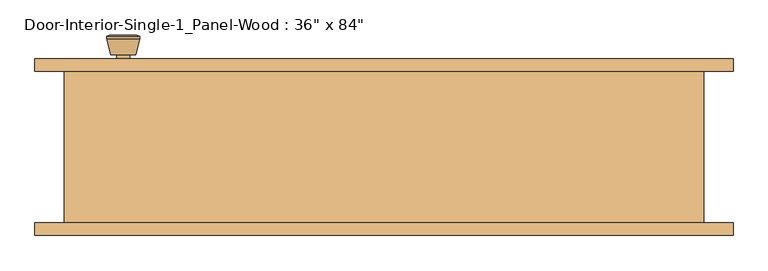
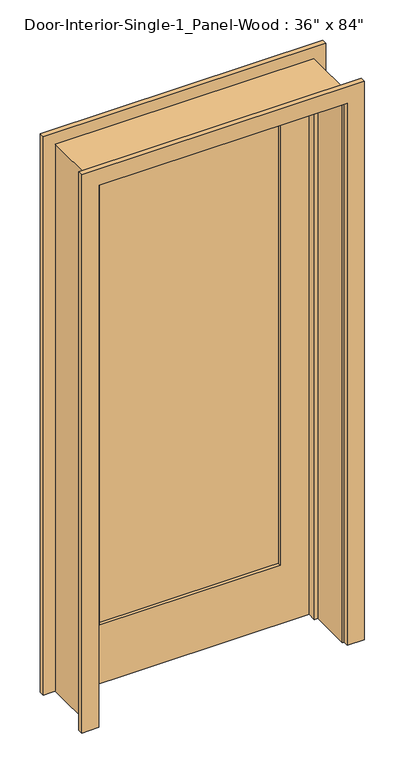
"""IFC4 building model written with IfcOpenShell, lengths in millimetres: door geometry."""

from ifc_helpers import new_model, si_unit, point, frame, frame_2d, origin, place, context, project, spatial, polyline, circle_curve, trimmed, segment, composite_curve, outline, extrude, faceted_brep, source, transform, mapped, element, save
from ifc_brep_helpers import plane_surface, cylinder_surface, revolved_surface, advanced_brep


def door_3b97b8e7(model_context):
    return source(origin(), model_context, "Body", "SolidModel", [
        advanced_brep(
        [(-393.7, 70.2, 914.4), (-383.7, 70.2, 914.4), (-403.7, 70.2, 914.4), (-373.2241324, 21.2, 914.4), (-393.7, 21.2, 914.4), (-414.1758676, 21.2, 914.4), (-368.7, 23.0278681, 914.4), (-418.7, 23.0278681, 914.4), (-368.7, 26.4915463, 914.4), (-418.7, 26.4915463, 914.4), (-375.063764, 51.2, 914.4), (-412.336236, 51.2, 914.4), (-383.7, 51.2, 914.4), (-403.7, 51.2, 914.4)],
        [
            (0, 1),
            (1, 2, circle_curve(frame((-393.7, 70.2, 914.4), z_axis=(0.0, 1.0, 0.0), x_axis=(-1.0, 0.0, 0.0)), 10.0)),
            (2, 0),
            (2, 1, circle_curve(frame((-393.7, 70.2, 914.4), z_axis=(0.0, 1.0, 0.0), x_axis=(-1.0, 0.0, 0.0)), 10.0)),
            (3, 4),
            (4, 5),
            (5, 3, circle_curve(frame((-393.7, 21.2, 914.4), z_axis=(0.0, -1.0, 0.0), x_axis=(-1.0, 0.0, 0.0)), 20.4758676)),
            (3, 5, circle_curve(frame((-393.7, 21.2, 914.4), z_axis=(0.0, -1.0, 0.0), x_axis=(-1.0, 0.0, 0.0)), 20.4758676)),
            (6, 3),
            (5, 7),
            (7, 6, circle_curve(frame((-393.7, 23.0278681, 914.4), z_axis=(0.0, -1.0, 0.0), x_axis=(-1.0, 0.0, 0.0)), 25.0)),
            (6, 7, circle_curve(frame((-393.7, 23.0278681, 914.4), z_axis=(0.0, -1.0, 0.0), x_axis=(-1.0, 0.0, 0.0)), 25.0)),
            (8, 6),
            (7, 9),
            (9, 8, circle_curve(frame((-393.7, 26.4915463, 914.4), z_axis=(0.0, -1.0, 0.0), x_axis=(-1.0, 0.0, 0.0)), 25.0)),
            (8, 9, circle_curve(frame((-393.7, 26.4915463, 914.4), z_axis=(0.0, -1.0, 0.0), x_axis=(-1.0, 0.0, 0.0)), 25.0)),
            (10, 8),
            (9, 11),
            (11, 10, circle_curve(frame((-393.7, 51.2, 914.4), z_axis=(0.0, -1.0, 0.0), x_axis=(-1.0, 0.0, 0.0)), 18.636236)),
            (10, 11, circle_curve(frame((-393.7, 51.2, 914.4), z_axis=(0.0, -1.0, 0.0), x_axis=(-1.0, 0.0, 0.0)), 18.636236)),
            (12, 10),
            (11, 13),
            (13, 12, circle_curve(frame((-393.7, 51.2, 914.4), z_axis=(0.0, -1.0, 0.0), x_axis=(-1.0, 0.0, 0.0)), 10.0)),
            (12, 13, circle_curve(frame((-393.7, 51.2, 914.4), z_axis=(0.0, -1.0, 0.0), x_axis=(-1.0, 0.0, 0.0)), 10.0)),
            (1, 12),
            (13, 2),
        ],
        [
            plane_surface(frame((-393.7, 70.2, 914.4), z_axis=(0.0, 1.0, 0.0), x_axis=(-1.0, 0.0, 0.0))),
            plane_surface(frame((-393.7, 21.2, 914.4), z_axis=(0.0, -1.0, 0.0), x_axis=(-1.0, 0.0, 0.0))),
            revolved_surface(polyline([(-414.1758676, 21.2, 914.4), (-418.7, 23.0278681, 914.4)]), (-393.7, 70.2, 914.4), (0.0, 1.0, 0.0)),
            cylinder_surface(frame((-393.7, 70.2, 914.4), z_axis=(0.0, 1.0, 0.0), x_axis=(-1.0, 0.0, 0.0)), 25.0),
            revolved_surface(polyline([(-418.7, 26.4915463, 914.4), (-412.336236, 51.2, 914.4)]), (-393.7, 70.2, 914.4), (0.0, 1.0, 0.0)),
            plane_surface(frame((-393.7, 51.2, 914.4), z_axis=(0.0, 1.0, 0.0), x_axis=(-1.0, 0.0, 0.0))),
            cylinder_surface(frame((-393.7, 70.2, 914.4), z_axis=(0.0, 1.0, 0.0), x_axis=(-1.0, 0.0, 0.0)), 10.0),
        ],
        [
            (0, [[1, 2, 3]]),
            (0, [[-3, 4, -1]]),
            (1, [[5, 6, 7]]),
            (1, [[-6, -5, 8]]),
            (2, [[9, -7, 10, 11]]),
            (2, [[-10, -8, -9, 12]]),
            (3, [[13, -11, 14, 15]]),
            (3, [[-14, -12, -13, 16]]),
            (4, [[17, -15, 18, 19]]),
            (4, [[-18, -16, -17, 20]]),
            (5, [[21, -19, 22, 23]]),
            (5, [[-22, -20, -21, 24]]),
            (6, [[25, -23, 26, -2]]),
            (6, [[-26, -24, -25, -4]]),
        ],
    ),
        extrude(outline(composite_curve([segment(trimmed(circle_curve(frame_2d((914.4, -393.7)), 30.0), [point((914.4, -423.7))], [point((914.4, -363.7))], False, "CARTESIAN"), True, "CONTINUOUS"), segment(trimmed(circle_curve(frame_2d((914.4, -393.7)), 30.0), [point((914.4, -363.7))], [point((914.4, -423.7))], False, "CARTESIAN"), True, "CONTINUOUS")], self_intersect=False)), frame((0.0, 70.2, 0.0), z_axis=(0.0, 1.0, 0.0), x_axis=(0.0, 0.0, 1.0)), (0.0, 0.0, 1.0), 6.0),
        advanced_brep(
        [(-393.7, 117.125, 914.4), (-403.7, 117.125, 914.4), (-383.7, 117.125, 914.4), (-373.2241324, 166.125, 914.4), (-414.1758676, 166.125, 914.4), (-393.7, 166.125, 914.4), (-368.7, 164.2971319, 914.4), (-418.7, 164.2971319, 914.4), (-368.7, 160.8334537, 914.4), (-418.7, 160.8334537, 914.4), (-375.063764, 136.125, 914.4), (-412.336236, 136.125, 914.4), (-383.7, 136.125, 914.4), (-403.7, 136.125, 914.4)],
        [
            (0, 1),
            (1, 2, circle_curve(frame((-393.7, 117.125, 914.4), z_axis=(0.0, -1.0, 0.0), x_axis=(-1.0, 0.0, 0.0)), 10.0)),
            (2, 0),
            (2, 1, circle_curve(frame((-393.7, 117.125, 914.4), z_axis=(0.0, -1.0, 0.0), x_axis=(-1.0, 0.0, 0.0)), 10.0)),
            (3, 4, circle_curve(frame((-393.7, 166.125, 914.4), z_axis=(0.0, 1.0, 0.0), x_axis=(-1.0, 0.0, 0.0)), 20.4758676)),
            (4, 5),
            (5, 3),
            (4, 3, circle_curve(frame((-393.7, 166.125, 914.4), z_axis=(0.0, 1.0, 0.0), x_axis=(-1.0, 0.0, 0.0)), 20.4758676)),
            (6, 7, circle_curve(frame((-393.7, 164.2971319, 914.4), z_axis=(0.0, 1.0, 0.0), x_axis=(-1.0, 0.0, 0.0)), 25.0)),
            (7, 4),
            (3, 6),
            (7, 6, circle_curve(frame((-393.7, 164.2971319, 914.4), z_axis=(0.0, 1.0, 0.0), x_axis=(-1.0, 0.0, 0.0)), 25.0)),
            (8, 9, circle_curve(frame((-393.7, 160.8334537, 914.4), z_axis=(0.0, 1.0, 0.0), x_axis=(-1.0, 0.0, 0.0)), 25.0)),
            (9, 7),
            (6, 8),
            (9, 8, circle_curve(frame((-393.7, 160.8334537, 914.4), z_axis=(0.0, 1.0, 0.0), x_axis=(-1.0, 0.0, 0.0)), 25.0)),
            (10, 11, circle_curve(frame((-393.7, 136.125, 914.4), z_axis=(0.0, 1.0, 0.0), x_axis=(-1.0, 0.0, 0.0)), 18.636236)),
            (11, 9),
            (8, 10),
            (11, 10, circle_curve(frame((-393.7, 136.125, 914.4), z_axis=(0.0, 1.0, 0.0), x_axis=(-1.0, 0.0, 0.0)), 18.636236)),
            (12, 13, circle_curve(frame((-393.7, 136.125, 914.4), z_axis=(0.0, 1.0, 0.0), x_axis=(-1.0, 0.0, 0.0)), 10.0)),
            (13, 11),
            (10, 12),
            (13, 12, circle_curve(frame((-393.7, 136.125, 914.4), z_axis=(0.0, 1.0, 0.0), x_axis=(-1.0, 0.0, 0.0)), 10.0)),
            (1, 13),
            (12, 2),
        ],
        [
            plane_surface(frame((-393.7, 117.125, 914.4), z_axis=(0.0, -1.0, 0.0), x_axis=(-1.0, 0.0, 0.0))),
            plane_surface(frame((-393.7, 166.125, 914.4), z_axis=(0.0, 1.0, 0.0), x_axis=(-1.0, 0.0, 0.0))),
            revolved_surface(polyline([(-414.1758676, 166.125, 914.4), (-418.7, 164.2971319, 914.4)]), (-393.7, 117.125, 914.4), (0.0, -1.0, 0.0)),
            cylinder_surface(frame((-393.7, 117.125, 914.4), z_axis=(0.0, -1.0, 0.0), x_axis=(-1.0, 0.0, 0.0)), 25.0),
            revolved_surface(polyline([(-418.7, 160.8334537, 914.4), (-412.336236, 136.125, 914.4)]), (-393.7, 117.125, 914.4), (0.0, -1.0, 0.0)),
            plane_surface(frame((-393.7, 136.125, 914.4), z_axis=(0.0, -1.0, 0.0), x_axis=(-1.0, 0.0, 0.0))),
            cylinder_surface(frame((-393.7, 117.125, 914.4), z_axis=(0.0, -1.0, 0.0), x_axis=(-1.0, 0.0, 0.0)), 10.0),
        ],
        [
            (0, [[1, 2, 3]]),
            (0, [[-3, 4, -1]]),
            (1, [[5, 6, 7]]),
            (1, [[8, -7, -6]]),
            (2, [[9, 10, -5, 11]]),
            (2, [[12, -11, -8, -10]]),
            (3, [[13, 14, -9, 15]]),
            (3, [[16, -15, -12, -14]]),
            (4, [[17, 18, -13, 19]]),
            (4, [[20, -19, -16, -18]]),
            (5, [[21, 22, -17, 23]]),
            (5, [[24, -23, -20, -22]]),
            (6, [[-2, 25, -21, 26]]),
            (6, [[-4, -26, -24, -25]]),
        ],
    ),
        extrude(outline(composite_curve([segment(trimmed(circle_curve(frame_2d((914.4, -393.7)), 30.0), [point((914.4, -423.7))], [point((914.4, -363.7))], False, "CARTESIAN"), True, "CONTINUOUS"), segment(trimmed(circle_curve(frame_2d((914.4, -393.7)), 30.0), [point((914.4, -363.7))], [point((914.4, -423.7))], False, "CARTESIAN"), True, "CONTINUOUS")], self_intersect=False)), frame((0.0, 111.125, 0.0), z_axis=(0.0, 1.0, 0.0), x_axis=(0.0, 0.0, 1.0)), (0.0, 0.0, 1.0), 6.0),
        faceted_brep([(482.6, 111.125, 0.0), (482.6, -117.475, 0.0), (457.2, -117.475, 0.0), (457.2, 41.275, 0.0), (444.5, 41.275, 0.0), (444.5, 76.2, 0.0), (457.2, 76.2, 0.0), (457.2, 111.125, 0.0), (482.6, 111.125, 2159.0), (482.6, -117.475, 2159.0), (-482.6, -117.475, 2159.0), (-482.6, -117.475, 0.0), (-457.2, -117.475, 0.0), (-457.2, -117.475, 2133.6), (457.2, -117.475, 2133.6), (457.2, 41.275, 2133.6), (-457.2, 41.275, 2133.6), (-457.2, 41.275, 0.0), (-444.5, 41.275, 0.0), (-444.5, 41.275, 2120.9), (444.5, 41.275, 2120.9), (444.5, 76.2, 2120.9), (-444.5, 76.2, 2120.9), (-444.5, 76.2, 0.0), (-457.2, 76.2, 0.0), (-457.2, 76.2, 2133.6), (457.2, 76.2, 2133.6), (457.2, 111.125, 2133.6), (-457.2, 111.125, 2133.6), (-457.2, 111.125, 0.0), (-482.6, 111.125, 0.0), (-482.6, 111.125, 2159.0)], [[[0, 1, 2, 3, 4, 5, 6, 7]], [[1, 0, 8, 9]], [[2, 1, 9, 10, 11, 12, 13, 14]], [[3, 2, 14, 15]], [[4, 3, 15, 16, 17, 18, 19, 20]], [[5, 4, 20, 21]], [[6, 5, 21, 22, 23, 24, 25, 26]], [[7, 6, 26, 27]], [[0, 7, 27, 28, 29, 30, 31, 8]], [[9, 8, 31, 10]], [[15, 14, 13, 16]], [[21, 20, 19, 22]], [[27, 26, 25, 28]], [[30, 29, 24, 23, 18, 17, 12, 11]], [[10, 31, 30, 11]], [[16, 13, 12, 17]], [[22, 19, 18, 23]], [[28, 25, 24, 29]]]),
        extrude(outline(polyline([(2133.6, -457.2), (0.0, -457.2), (0.0, 457.2), (2133.6, 457.2), (2133.6, -457.2)]), holes=[polyline([(2014.5375, -336.55), (2014.5375, 336.55), (231.775, 336.55), (231.775, -336.55), (2014.5375, -336.55)])]), frame((0.0, 76.2, 0.0), z_axis=(0.0, 1.0, 0.0), x_axis=(0.0, 0.0, 1.0)), (0.0, 0.0, 1.0), 34.925),
        extrude(outline(polyline([(336.55, 87.8416667), (-336.55, 87.8416667), (-336.55, 99.4833333), (336.55, 99.4833333), (336.55, 87.8416667)])), frame((0.0, 0.0, 231.775), z_axis=(0.0, 0.0, 1.0), x_axis=(1.0, 0.0, 0.0)), (0.0, 0.0, 1.0), 1782.7625),
        extrude(outline(polyline([(0.0, 463.55), (0.0, 527.05), (2203.45, 527.05), (2203.45, -527.05), (0.0, -527.05), (0.0, -463.55), (2139.95, -463.55), (2139.95, 463.55), (0.0, 463.55)])), frame((0.0, 111.125, 0.0), z_axis=(0.0, 1.0, 0.0), x_axis=(0.0, 0.0, 1.0)), (0.0, 0.0, 1.0), 19.05),
        extrude(outline(polyline([(0.0, 463.55), (0.0, 527.05), (2203.45, 527.05), (2203.45, -527.05), (0.0, -527.05), (0.0, -463.55), (2139.95, -463.55), (2139.95, 463.55), (0.0, 463.55)])), frame((0.0, -136.525, 0.0), z_axis=(0.0, 1.0, 0.0), x_axis=(0.0, 0.0, 1.0)), (0.0, 0.0, 1.0), 19.05),
    ])


if __name__ == "__main__":
    model = new_model("IFC4")
    model_context = context("Model", 3, world=origin())
    ifc_project = project(units=[si_unit("LENGTHUNIT", "METRE", prefix="MILLI")], contexts=[model_context])
    site = spatial("IfcSite", under=ifc_project)
    building = spatial("IfcBuilding", under=site)
    placement = place(None, origin())
    door_shape = door_3b97b8e7(model_context)
    element("IfcDoor", 1, ObjectType="Door-Interior-Single-1_Panel-Wood : 36\" x 84\"", at=placement, inside=building, context=model_context, shape_type="MappedRepresentation", body=[
        mapped(door_shape, transform((0.0, 0.0, 0.0), x_axis=(1.0, 0.0, 0.0), y_axis=(0.0, 1.0, 0.0), z_axis=(0.0, 0.0, 1.0))),
    ])
    save(model, "model.ifc")

# Revit data of these elements
# Type "Door-Interior-Single-1_Panel-Wood : 36\" x 84\""
#   Type Mark = "8"
#   Assembly Code = "C1020300"
#   Analytic Construction = "Wooden"
#   Top Rail = 0' - 4 11/16"
#   Thickness = 0' - 1 3/8"
#   Thermal Resistance (R) = 2.5876 (h·ft²·°F)/BTU
#   Swing Angle [instance default] = 90.00°
#   Stiles = 0' - 4 3/4"
#   Rough Width = 3' - 2"
#   Rough Height = 7' - 1"
#   Height = 7' - 0"
#   Width = 3' - 0"
#   Heat Transfer Coefficient (U) = 0.3865 BTU/(h·ft²·°F)
#   Bottom Rail = 0' - 9 1/8"
#   Panel Material = door colour
#   Frame Material = door colour
#   Door Handle Material = door colour
#   Visual Light Transmittance = 0
#   Solar Heat Gain Coefficient = 0
#   Wall Closure = (empty or 0)
#   Function = (empty or 0)
# Element 1 (IfcDoor, "Door-Interior-Single-1_Panel-Wood : 36\" x 84\"")
#   Materials on its faces: "door colour"
# Materials
#   "door colour": class "Generic", colour RGB 120 120 120, transparency 0, Cost = 0
